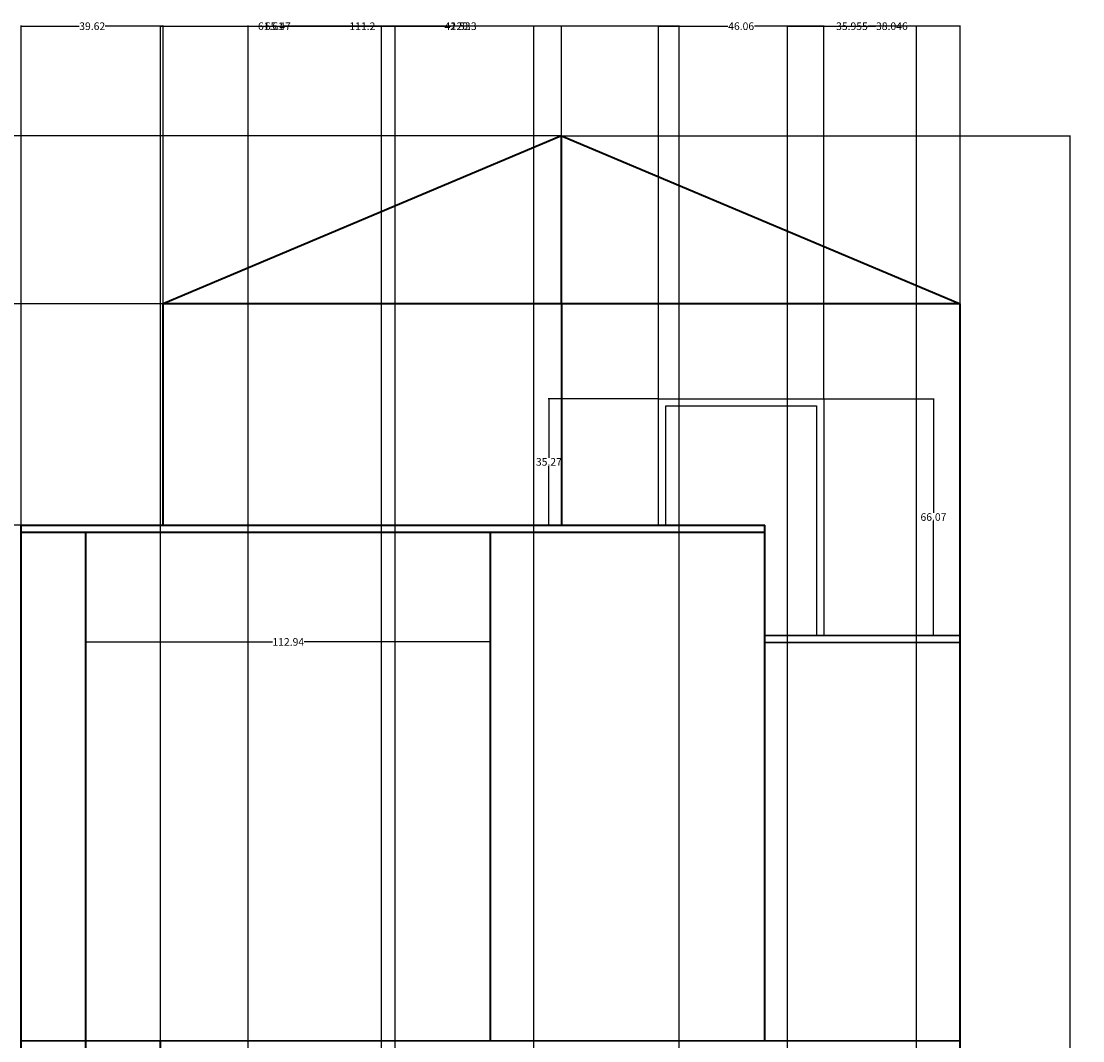
# Model space of a CAD drawing. Units: inches. Extents: x -113 to 379, y 13 to 689.
# Tile 5 of 5: x 82 to 378, y 405 to 689. Entities that reach past the tile are written whole.
import ezdxf

# ---------------------------------------------------------------- set-up
doc = ezdxf.new("R2010")
doc.units = ezdxf.units.IN
doc.header["$MEASUREMENT"] = 0
for name, color, linetype, lineweight in [('A-ANNO-DIMS', 2, 'Continuous', 18), ('A-DOOR', 3, 'Continuous', 25), ('A-FLOR', 7, 'Continuous', 30), ('A-ROOF', 1, 'Continuous', 35), ('A-WALL', 7, 'Continuous', 35)]:
    doc.layers.add(name, color=color, linetype=linetype, lineweight=lineweight)
doc.styles.get("Standard").update_dxf_attribs({"font": 'arial.ttf'})
doc.dimstyles.get("Standard").update_dxf_attribs({"dimtxt": 2.125, "dimasz": 0.18, "dimexe": 0.18, "dimexo": 0.0625, "dimgap": 0.09, "dimtad": 0, "dimtih": 1, "dimtoh": 1, "dimdec": 4, "dimzin": 0, "dimdsep": 46, "dimlunit": 4, "dimtxsty": 'Standard', "dimcen": 0.09, "dimadec": 0, "dimazin": 0, "dimtfac": 1, "dimtdec": 4, "dimtofl": 0, "dimtmove": 0, "dimatfit": 3, "dimfxl": 1, "dimtolj": 1, "dimtzin": 0, "dimarcsym": 0})

# ---------------------------------------------------------------- blocks, each defined once
blk = doc.blocks.new('*D20')
at = {"layer": 'A-ANNO-DIMS', "color": 0, "lineweight": -2, "transparency": 16777216}
for p, q in [((232.74, 657.3), (374.68, 657.3)), ((374.5, 657.12), (374.5, 388.15)), ((374.5, 116.83), (374.5, 385.8)), ((343.93, 116.65), (374.68, 116.65))]:
    blk.add_line(p, q, dxfattribs=at)
at = {"layer": 'A-ANNO-DIMS', "color": 0, "transparency": 16777216}
for points in [[(374.47, 657.12), (374.53, 657.12), (374.5, 657.3)], [(374.47, 116.83), (374.53, 116.83), (374.5, 116.65)]]:
    blk.add_solid(points, dxfattribs=at)
at = {"layer": 'Defpoints', "color": 0, "transparency": 16777216}
for p in [(232.68, 657.3), (374.5, 657.3), (343.87, 116.65)]:
    blk.add_point(p, dxfattribs=at)
at = {"layer": 'A-ANNO-DIMS', "color": 0, "transparency": 16777216, "insert": (374.5, 386.98), "char_height": 2.125, "attachment_point": 5}
blk.add_mtext('\\A1;540.7', dxfattribs=at)
blk = doc.blocks.new('*D21')
at = {"layer": 'A-ANNO-DIMS', "color": 0, "lineweight": -2, "transparency": 16777216}
for p, q in [((232.62, 657.3), (-108.66, 657.3)), ((-108.48, 657.12), (-108.48, 635.04)), ((-108.48, 610.6), (-108.48, 632.69)), ((121.43, 610.42), (-108.66, 610.42))]:
    blk.add_line(p, q, dxfattribs=at)
at = {"layer": 'A-ANNO-DIMS', "color": 0, "transparency": 16777216}
for points in [[(-108.51, 657.12), (-108.45, 657.12), (-108.48, 657.3)], [(-108.51, 610.6), (-108.45, 610.6), (-108.48, 610.42)]]:
    blk.add_solid(points, dxfattribs=at)
at = {"layer": 'Defpoints', "color": 0, "transparency": 16777216}
for p in [(-108.48, 657.3), (232.68, 657.3), (121.49, 610.42)]:
    blk.add_point(p, dxfattribs=at)
at = {"layer": 'A-ANNO-DIMS', "color": 0, "transparency": 16777216, "insert": (-108.48, 633.86), "char_height": 2.125, "attachment_point": 5}
blk.add_mtext('\\A1;46.88', dxfattribs=at)
blk = doc.blocks.new('*D22')
at = {"layer": 'A-ANNO-DIMS', "color": 0, "lineweight": -2, "transparency": 16777216}
for p, q in [((121.49, 610.48), (121.49, 688.12)), ((121.67, 687.94), (173.52, 687.94)), ((232.5, 687.94), (180.65, 687.94)), ((232.68, 657.36), (232.68, 688.12))]:
    blk.add_line(p, q, dxfattribs=at)
at = {"layer": 'A-ANNO-DIMS', "color": 0, "transparency": 16777216}
for points in [[(121.67, 687.97), (121.67, 687.91), (121.49, 687.94)], [(232.5, 687.97), (232.5, 687.91), (232.68, 687.94)]]:
    blk.add_solid(points, dxfattribs=at)
at = {"layer": 'Defpoints', "color": 0, "transparency": 16777216}
for p in [(232.68, 687.94), (232.68, 657.3), (121.49, 610.42)]:
    blk.add_point(p, dxfattribs=at)
at = {"layer": 'A-ANNO-DIMS', "color": 0, "transparency": 16777216, "insert": (177.08, 687.94), "char_height": 2.125, "attachment_point": 5}
blk.add_mtext('\\A1;111.2', dxfattribs=at)
blk = doc.blocks.new('*D23')
at = {"layer": 'A-ANNO-DIMS', "color": 0, "lineweight": -2, "transparency": 16777216}
for p, q in [((81.87, 548.71), (81.87, 688.12)), ((82.05, 687.94), (98.02, 687.94)), ((121.31, 687.94), (105.34, 687.94)), ((121.49, 610.48), (121.49, 688.12))]:
    blk.add_line(p, q, dxfattribs=at)
at = {"layer": 'A-ANNO-DIMS', "color": 0, "transparency": 16777216}
for points in [[(82.05, 687.97), (82.05, 687.91), (81.87, 687.94)], [(121.31, 687.97), (121.31, 687.91), (121.49, 687.94)]]:
    blk.add_solid(points, dxfattribs=at)
at = {"layer": 'Defpoints', "color": 0, "transparency": 16777216}
for p in [(121.49, 687.94), (121.49, 610.42), (81.87, 548.65)]:
    blk.add_point(p, dxfattribs=at)
at = {"layer": 'A-ANNO-DIMS', "color": 0, "transparency": 16777216, "insert": (101.68, 687.94), "char_height": 2.125, "attachment_point": 5}
blk.add_mtext('\\A1;39.62', dxfattribs=at)
blk = doc.blocks.new('*D24')
at = {"layer": 'A-ANNO-DIMS', "color": 0, "lineweight": -2, "transparency": 16777216}
for p, q in [((259.76, 583.98), (259.76, 688.12)), ((259.94, 687.94), (279.08, 687.94)), ((305.64, 687.94), (286.51, 687.94)), ((305.82, 583.98), (305.82, 688.12))]:
    blk.add_line(p, q, dxfattribs=at)
at = {"layer": 'A-ANNO-DIMS', "color": 0, "transparency": 16777216}
for points in [[(259.94, 687.97), (259.94, 687.91), (259.76, 687.94)], [(305.64, 687.97), (305.64, 687.91), (305.82, 687.94)]]:
    blk.add_solid(points, dxfattribs=at)
at = {"layer": 'Defpoints', "color": 0, "transparency": 16777216}
for p in [(305.82, 687.94), (259.76, 583.92), (305.82, 583.92)]:
    blk.add_point(p, dxfattribs=at)
at = {"layer": 'A-ANNO-DIMS', "color": 0, "transparency": 16777216, "insert": (282.79, 687.94), "char_height": 2.125, "attachment_point": 5}
blk.add_mtext('\\A1;46.06', dxfattribs=at)
blk = doc.blocks.new('*D25')
at = {"layer": 'A-ANNO-DIMS', "color": 0, "lineweight": -2, "transparency": 16777216}
for p, q in [((305.82, 583.98), (305.82, 688.12)), ((306, 687.94), (320.35, 687.94)), ((343.69, 687.94), (329.35, 687.94)), ((343.87, 610.48), (343.87, 688.12))]:
    blk.add_line(p, q, dxfattribs=at)
at = {"layer": 'A-ANNO-DIMS', "color": 0, "transparency": 16777216}
for points in [[(306, 687.97), (306, 687.91), (305.82, 687.94)], [(343.69, 687.97), (343.69, 687.91), (343.87, 687.94)]]:
    blk.add_solid(points, dxfattribs=at)
at = {"layer": 'Defpoints', "color": 0, "transparency": 16777216}
for p in [(343.87, 687.94), (343.87, 610.42), (305.82, 583.92)]:
    blk.add_point(p, dxfattribs=at)
at = {"layer": 'A-ANNO-DIMS', "color": 0, "transparency": 16777216, "insert": (324.85, 687.94), "char_height": 2.125, "attachment_point": 5}
blk.add_mtext('\\A1;38.046', dxfattribs=at)
blk = doc.blocks.new('*D26')
at = {"layer": 'A-ANNO-DIMS', "color": 0, "lineweight": -2, "transparency": 16777216}
for p, q in [((259.7, 583.92), (228.95, 583.92)), ((229.13, 583.74), (229.13, 567.46)), ((229.13, 548.83), (229.13, 565.11)), ((259.7, 548.65), (228.95, 548.65))]:
    blk.add_line(p, q, dxfattribs=at)
at = {"layer": 'A-ANNO-DIMS', "color": 0, "transparency": 16777216}
for points in [[(229.1, 583.74), (229.16, 583.74), (229.13, 583.92)], [(229.1, 548.83), (229.16, 548.83), (229.13, 548.65)]]:
    blk.add_solid(points, dxfattribs=at)
at = {"layer": 'Defpoints', "color": 0, "transparency": 16777216}
for p in [(229.13, 583.92), (259.76, 583.92), (259.76, 548.65)]:
    blk.add_point(p, dxfattribs=at)
at = {"layer": 'A-ANNO-DIMS', "color": 0, "transparency": 16777216, "insert": (229.13, 566.29), "char_height": 2.125, "attachment_point": 5}
blk.add_mtext('\\A1;35.27', dxfattribs=at)
blk = doc.blocks.new('*D27')
at = {"layer": 'A-ANNO-DIMS', "color": 0, "lineweight": -2, "transparency": 16777216}
for p, q in [((305.89, 583.92), (336.64, 583.92)), ((336.46, 583.74), (336.46, 552.06)), ((336.46, 518.03), (336.46, 549.71)), ((305.89, 517.85), (336.64, 517.85))]:
    blk.add_line(p, q, dxfattribs=at)
at = {"layer": 'A-ANNO-DIMS', "color": 0, "transparency": 16777216}
for points in [[(336.43, 583.74), (336.49, 583.74), (336.46, 583.92)], [(336.43, 518.03), (336.49, 518.03), (336.46, 517.85)]]:
    blk.add_solid(points, dxfattribs=at)
at = {"layer": 'Defpoints', "color": 0, "transparency": 16777216}
for p in [(305.82, 583.92), (305.82, 517.85), (336.46, 517.85)]:
    blk.add_point(p, dxfattribs=at)
at = {"layer": 'A-ANNO-DIMS', "color": 0, "transparency": 16777216, "insert": (336.46, 550.89), "char_height": 2.125, "attachment_point": 5}
blk.add_mtext('\\A1;66.07', dxfattribs=at)
blk = doc.blocks.new('*D28')
at = {"layer": 'A-ANNO-DIMS', "color": 0, "lineweight": -2, "transparency": 16777216}
for p, q in [((121.43, 610.42), (-108.66, 610.42)), ((-108.48, 610.24), (-108.48, 580.71)), ((-108.48, 548.83), (-108.48, 578.36)), ((81.81, 548.65), (-108.66, 548.65))]:
    blk.add_line(p, q, dxfattribs=at)
at = {"layer": 'A-ANNO-DIMS', "color": 0, "transparency": 16777216}
for points in [[(-108.51, 610.24), (-108.45, 610.24), (-108.48, 610.42)], [(-108.51, 548.83), (-108.45, 548.83), (-108.48, 548.65)]]:
    blk.add_solid(points, dxfattribs=at)
at = {"layer": 'Defpoints', "color": 0, "transparency": 16777216}
for p in [(-108.48, 610.42), (121.49, 610.42), (81.87, 548.65)]:
    blk.add_point(p, dxfattribs=at)
at = {"layer": 'A-ANNO-DIMS', "color": 0, "transparency": 16777216, "insert": (-108.48, 579.54), "char_height": 2.125, "attachment_point": 5}
blk.add_mtext('\\A1;61.77', dxfattribs=at)
blk = doc.blocks.new('*D32')
at = {"layer": 'A-ANNO-DIMS', "color": 0, "lineweight": -2, "transparency": 16777216}
for p, q in [((99.93, 546.59), (99.93, 515.84)), ((212.87, 546.59), (212.87, 515.84)), ((100.11, 516.02), (152.01, 516.02)), ((212.69, 516.02), (160.8, 516.02))]:
    blk.add_line(p, q, dxfattribs=at)
at = {"layer": 'A-ANNO-DIMS', "color": 0, "transparency": 16777216}
for points in [[(100.11, 516.05), (100.11, 515.99), (99.93, 516.02)], [(212.69, 516.05), (212.69, 515.99), (212.87, 516.02)]]:
    blk.add_solid(points, dxfattribs=at)
at = {"layer": 'Defpoints', "color": 0, "transparency": 16777216}
for p in [(99.93, 546.65), (212.87, 546.65), (99.93, 516.02)]:
    blk.add_point(p, dxfattribs=at)
at = {"layer": 'A-ANNO-DIMS', "color": 0, "transparency": 16777216, "insert": (156.4, 516.02), "char_height": 2.125, "attachment_point": 5}
blk.add_mtext('\\A1;112.94', dxfattribs=at)
blk = doc.blocks.new('*D33')
at = {"layer": 'A-ANNO-DIMS', "color": 0, "lineweight": -2, "transparency": 16777216}
for p, q in [((120.75, 221.89), (120.75, 688.12)), ((120.93, 687.94), (149.81, 687.94)), ((186.04, 687.94), (157.17, 687.94)), ((186.22, 221.89), (186.22, 688.12))]:
    blk.add_line(p, q, dxfattribs=at)
at = {"layer": 'A-ANNO-DIMS', "color": 0, "transparency": 16777216}
for points in [[(120.93, 687.97), (120.93, 687.91), (120.75, 687.94)], [(186.04, 687.97), (186.04, 687.91), (186.22, 687.94)]]:
    blk.add_solid(points, dxfattribs=at)
at = {"layer": 'Defpoints', "color": 0, "transparency": 16777216}
for p in [(186.22, 687.94), (120.75, 221.82), (186.22, 221.82)]:
    blk.add_point(p, dxfattribs=at)
at = {"layer": 'A-ANNO-DIMS', "color": 0, "transparency": 16777216, "insert": (153.49, 687.94), "char_height": 2.125, "attachment_point": 5}
blk.add_mtext('\\A1;65.47', dxfattribs=at)
blk = doc.blocks.new('*D39')
at = {"layer": 'A-ANNO-DIMS', "color": 0, "lineweight": -2, "transparency": 16777216}
for p, q in [((145.2, 370.61), (145.2, 688.12)), ((145.38, 687.94), (201.77, 687.94)), ((265.31, 687.94), (208.92, 687.94)), ((265.49, 370.61), (265.49, 688.12))]:
    blk.add_line(p, q, dxfattribs=at)
at = {"layer": 'A-ANNO-DIMS', "color": 0, "transparency": 16777216}
for points in [[(145.38, 687.97), (145.38, 687.91), (145.2, 687.94)], [(265.31, 687.97), (265.31, 687.91), (265.49, 687.94)]]:
    blk.add_solid(points, dxfattribs=at)
at = {"layer": 'Defpoints', "color": 0, "transparency": 16777216}
for p in [(265.49, 687.94), (145.2, 370.54), (265.49, 370.54)]:
    blk.add_point(p, dxfattribs=at)
at = {"layer": 'A-ANNO-DIMS', "color": 0, "transparency": 16777216, "insert": (205.34, 687.94), "char_height": 2.125, "attachment_point": 5}
blk.add_mtext('\\A1;120.3', dxfattribs=at)
blk = doc.blocks.new('*D42')
at = {"layer": 'A-ANNO-DIMS', "color": 0, "lineweight": -2, "transparency": 16777216}
for p, q in [((295.73, 389.63), (295.73, 688.12)), ((295.91, 687.94), (309.2, 687.94)), ((331.5, 687.94), (318.21, 687.94)), ((331.68, 389.63), (331.68, 688.12))]:
    blk.add_line(p, q, dxfattribs=at)
at = {"layer": 'A-ANNO-DIMS', "color": 0, "transparency": 16777216}
for points in [[(295.91, 687.97), (295.91, 687.91), (295.73, 687.94)], [(331.5, 687.97), (331.5, 687.91), (331.68, 687.94)]]:
    blk.add_solid(points, dxfattribs=at)
at = {"layer": 'Defpoints', "color": 0, "transparency": 16777216}
for p in [(331.68, 687.94), (295.73, 389.57), (331.68, 389.57)]:
    blk.add_point(p, dxfattribs=at)
at = {"layer": 'A-ANNO-DIMS', "color": 0, "transparency": 16777216, "insert": (313.71, 687.94), "char_height": 2.125, "attachment_point": 5}
blk.add_mtext('\\A1;35.955', dxfattribs=at)
blk = doc.blocks.new('*D58')
at = {"layer": 'A-ANNO-DIMS', "color": 0, "lineweight": -2, "transparency": 16777216}
for p, q in [((182.37, 329.3), (182.37, 688.12)), ((182.55, 687.94), (199.91, 687.94)), ((224.72, 687.94), (207.35, 687.94)), ((224.9, 329.3), (224.9, 688.12))]:
    blk.add_line(p, q, dxfattribs=at)
at = {"layer": 'A-ANNO-DIMS', "color": 0, "transparency": 16777216}
for points in [[(182.55, 687.97), (182.55, 687.91), (182.37, 687.94)], [(224.72, 687.97), (224.72, 687.91), (224.9, 687.94)]]:
    blk.add_solid(points, dxfattribs=at)
at = {"layer": 'Defpoints', "color": 0, "transparency": 16777216}
for p in [(224.9, 687.94), (182.37, 329.23), (224.9, 329.23)]:
    blk.add_point(p, dxfattribs=at)
at = {"layer": 'A-ANNO-DIMS', "color": 0, "transparency": 16777216, "insert": (203.63, 687.94), "char_height": 2.125, "attachment_point": 5}
blk.add_mtext('\\A1;42.53', dxfattribs=at)
blk = doc.blocks.new('*D59')
at = {"layer": 'A-ANNO-DIMS', "color": 0, "lineweight": -2, "transparency": 16777216}
for p, q in [((120.75, 329.3), (120.75, 688.12)), ((120.93, 687.94), (148.08, 687.94)), ((182.19, 687.94), (155.04, 687.94)), ((182.37, 329.3), (182.37, 688.12))]:
    blk.add_line(p, q, dxfattribs=at)
at = {"layer": 'A-ANNO-DIMS', "color": 0, "transparency": 16777216}
for points in [[(120.93, 687.97), (120.93, 687.91), (120.75, 687.94)], [(182.19, 687.97), (182.19, 687.91), (182.37, 687.94)]]:
    blk.add_solid(points, dxfattribs=at)
at = {"layer": 'Defpoints', "color": 0, "transparency": 16777216}
for p in [(182.37, 687.94), (120.75, 329.23), (182.37, 329.23)]:
    blk.add_point(p, dxfattribs=at)
at = {"layer": 'A-ANNO-DIMS', "color": 0, "transparency": 16777216, "insert": (151.56, 687.94), "char_height": 2.125, "attachment_point": 5}
blk.add_mtext('\\A1;61.61', dxfattribs=at)

msp = doc.modelspace()

# ---------------------------------------------------------------- linework, layer by layer
at = {"layer": 'A-DOOR'}
for p, q in [((259.7647, 548.6509), (259.7647, 583.9211)), ((259.7647, 583.9211), (305.8234, 583.9211)), ((305.8234, 583.9211), (305.8234, 517.8535)), ((261.7647, 581.9211), (303.8234, 581.9211)), ((261.7647, 548.6509), (261.7647, 581.9211)), ((303.8234, 581.9211), (303.8234, 517.8535))]:
    msp.add_line(p, q, dxfattribs=at)
at = {"layer": 'A-FLOR'}
for p, q in [((343.8693, 517.8535), (289.3958, 517.8535)), ((343.8693, 515.8535), (289.3958, 515.8535)), ((81.8721, 404.6509), (343.8693, 404.6509))]:
    msp.add_line(p, q, dxfattribs=at)
at = {"layer": 'A-ROOF'}
for p, q in [((232.6797, 657.3014), (121.4902, 610.4218)), ((232.6797, 610.4218), (232.6797, 657.3014)), ((232.6797, 657.3014), (343.8693, 610.4218)), ((343.8693, 610.4218), (121.4902, 610.4218)), ((81.8721, 548.6509), (289.3958, 548.6509)), ((81.8721, 546.6509), (289.3958, 546.6509))]:
    msp.add_line(p, q, dxfattribs=at)
at = {"layer": 'A-WALL'}
for p, q in [((121.4902, 548.6509), (121.4902, 610.4218)), ((232.6797, 610.4218), (232.6797, 548.6509)), ((343.8693, 509.7523), (343.8693, 610.4218)), ((81.8721, 404.6509), (81.8721, 548.6509)), ((289.3958, 404.6509), (289.3958, 548.6509)), ((99.9328, 404.6509), (99.9328, 546.6509)), ((212.8707, 404.6509), (212.8707, 546.6509)), ((343.8693, 404.6509), (343.8693, 509.7523)), ((81.8721, 260.6509), (81.8721, 404.6509)), ((99.9328, 260.6509), (99.9328, 404.6509)), ((120.7533, 260.6509), (120.7533, 404.6509)), ((343.8693, 260.6509), (343.8693, 404.6509))]:
    msp.add_line(p, q, dxfattribs=at)

# ---------------------------------------------------------------- dimensions: what is measured, and where the dimension line sits
at = {"layer": 'A-ANNO-DIMS'}
for base, p1, p2, override, picture, middle in [((121.4902, 687.9364), (81.8721, 548.6509), (121.4902, 610.4218), {"dimdec": 2, "dimlfac": 1, "dimrnd": 0, "dimzin": 0, "dimdsep": 46, "dimlunit": 2}, '*D23', (101.6811, 687.9364)), ((186.2204, 687.9364), (120.7533, 221.8228), (186.2204, 221.8228), {"dimdec": 2, "dimlfac": 1, "dimrnd": 0, "dimzin": 0, "dimdsep": 46, "dimlunit": 2}, '*D33', (153.4869, 687.9364)), ((182.3676, 687.9364), (120.7533, 329.234), (182.3676, 329.234), {"dimdec": 2, "dimlfac": 1, "dimrnd": 0, "dimzin": 0, "dimdsep": 46, "dimlunit": 2}, '*D59', (151.5604, 687.9364)), ((232.6797, 687.9364), (121.4902, 610.4218), (232.6797, 657.3014), {"dimdec": 1, "dimlfac": 1, "dimrnd": 0, "dimzin": 0, "dimdsep": 46, "dimlunit": 2}, '*D22', (177.0849, 687.9364)), ((265.4865, 687.9364), (145.1985, 370.5425), (265.4865, 370.5425), {"dimdec": 1, "dimlfac": 1, "dimrnd": 0, "dimzin": 0, "dimdsep": 46, "dimlunit": 2}, '*D39', (205.3425, 687.9364)), ((224.8984, 687.9364), (182.3676, 329.234), (224.8984, 329.234), {"dimdec": 2, "dimlfac": 1, "dimrnd": 0, "dimzin": 0, "dimdsep": 46, "dimlunit": 2}, '*D58', (203.633, 687.9364)), ((305.8234, 687.9364), (259.7647, 583.9211), (305.8234, 583.9211), {"dimdec": 2, "dimlfac": 1, "dimrnd": 0, "dimzin": 0, "dimdsep": 46, "dimlunit": 2}, '*D24', (282.7941, 687.9364)), ((331.6831, 687.9364), (295.728, 389.5666), (331.6831, 389.5666), {"dimdec": 3, "dimlfac": 1, "dimrnd": 0, "dimzin": 0, "dimdsep": 46, "dimlunit": 2}, '*D42', (313.7055, 687.9364)), ((343.8693, 687.9364), (305.8234, 583.9211), (343.8693, 610.4218), {"dimdec": 3, "dimlfac": 1, "dimrnd": 0, "dimzin": 0, "dimdsep": 46, "dimlunit": 2}, '*D25', (324.8464, 687.9364))]:
    dim = msp.add_linear_dim(base=base, p1=p1, p2=p2, dimstyle='Standard', override=override, dxfattribs=at)
    dim.commit()
    dim.dimension.update_dxf_attribs({"geometry": picture, "text_midpoint": middle})
for base, p1, p2, angle, override, picture, middle in [((-108.4772, 657.3014), (121.4902, 610.4218), (232.6797, 657.3014), 90, {"dimdec": 2, "dimlfac": 1, "dimrnd": 0, "dimzin": 0, "dimdsep": 46, "dimlunit": 2}, '*D21', (-108.4772, 633.8616)), ((374.5043, 657.3014), (343.8693, 116.6509), (232.6797, 657.3014), 90, {"dimdec": 1, "dimlfac": 1, "dimrnd": 0, "dimzin": 0, "dimdsep": 46, "dimlunit": 2}, '*D20', (374.5043, 386.9762)), ((-108.4772, 610.4218), (81.8721, 548.6509), (121.4902, 610.4218), 90, {"dimdec": 2, "dimlfac": 1, "dimrnd": 0, "dimzin": 0, "dimdsep": 46, "dimlunit": 2}, '*D28', (-108.4772, 579.5364)), ((229.1297, 583.9211), (259.7647, 548.6509), (259.7647, 583.9211), 90, {"dimdec": 2, "dimlfac": 1, "dimrnd": 0, "dimzin": 0, "dimdsep": 46, "dimlunit": 2}, '*D26', (229.1297, 566.286)), ((336.4584, 517.8535), (305.8234, 583.9211), (305.8234, 517.8535), 270, {"dimdec": 2, "dimlfac": 1, "dimrnd": 0, "dimzin": 0, "dimdsep": 46, "dimlunit": 2}, '*D27', (336.4584, 550.8873)), ((99.9328, 516.0159), (212.8707, 546.6509), (99.9328, 546.6509), 180, {"dimdec": 2, "dimlfac": 1, "dimrnd": 0, "dimzin": 0, "dimdsep": 46, "dimlunit": 2}, '*D32', (156.4018, 516.0159))]:
    dim = msp.add_linear_dim(base=base, p1=p1, p2=p2, angle=angle, dimstyle='Standard', override=override, dxfattribs=at)
    dim.commit()
    dim.dimension.update_dxf_attribs({"geometry": picture, "text_midpoint": middle})

doc.saveas('drawing.dxf')
